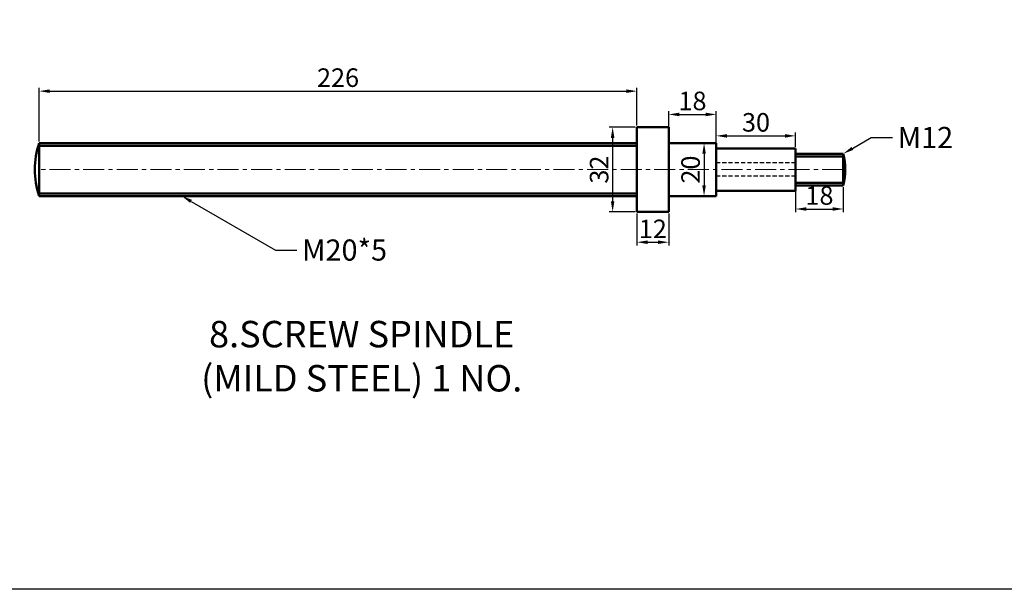
# Model space of a CAD drawing. Units: millimetres. Extents: x -66 to 1195, y -396 to 398.
# Tile 3 of 8: x 373 to 745, y -396 to -180. Entities that reach past the tile are written whole.
import ezdxf
from ezdxf import colors
from ezdxf.entities.mleader import LeaderData, LeaderLine
from ezdxf.math import Vec2, Vec3

# ---------------------------------------------------------------- set-up
doc = ezdxf.new("R2010")
doc.units = ezdxf.units.MM
doc.header["$LTSCALE"] = 0.5
doc.linetypes.add('CENTER', pattern=[50.8, 31.75, -6.35, 6.35, -6.35])
doc.linetypes.add('HIDDEN', pattern=[9.525, 6.35, -3.175])
for name, color, linetype, lineweight in [('M-CNTR', 1, 'CENTER', 18), ('M-DIMS', 2, 'Continuous', 25), ('M-HIDN', 3, 'HIDDEN', 25), ('M-OUTL', 7, 'Continuous', 50), ('M-TEXT', 7, 'Continuous', 25), ('M-TTLB', 7, 'Continuous', 25)]:
    doc.layers.add(name, color=color, linetype=linetype, lineweight=lineweight)
doc.styles.get("Standard").update_dxf_attribs({"font": 'arial.ttf'})
doc.dimstyles.new('ISO-25', dxfattribs={"dimtxt": 7, "dimasz": 4, "dimexe": 1.25, "dimexo": 0.625, "dimtad": 1, "dimtoh": 1, "dimtxsty": 'Standard', "dimcen": 2.5, "dimadec": 0, "dimazin": 0, "dimtfac": 1, "dimtmove": 0, "dimatfit": 3, "dimfxl": 1, "dimarcsym": 0})

# ---------------------------------------------------------------- blocks, each defined once
blk = doc.blocks.new('*D96')
at = {"layer": 'Defpoints', "color": 0, "ltscale": 0.5, "transparency": 16777216}
for p in [(606.02, -207.48), (606.02, -221.12), (380.02, -227.12)]:
    blk.add_point(p, dxfattribs=at)
at = {"layer": 'M-DIMS', "color": 0, "lineweight": -2, "ltscale": 0.5, "transparency": 16777216}
for p, q in [((380.02, -226.49), (380.02, -206.23)), ((384.02, -207.48), (602.02, -207.48)), ((606.02, -220.49), (606.02, -206.23))]:
    blk.add_line(p, q, dxfattribs=at)
at = {"layer": 'M-DIMS', "color": 0, "ltscale": 0.5, "transparency": 16777216}
for points in [[(384.02, -206.82), (384.02, -208.15), (380.02, -207.48)], [(602.02, -206.82), (602.02, -208.15), (606.02, -207.48)]]:
    blk.add_solid(points, dxfattribs=at)
at = {"layer": 'M-DIMS', "color": 0, "ltscale": 0.5, "transparency": 16777216, "insert": (493.02, -203.28), "char_height": 7, "attachment_point": 5}
blk.add_mtext('226', dxfattribs=at)
blk = doc.blocks.new('*D97')
at = {"layer": 'Defpoints', "color": 0, "ltscale": 0.5, "transparency": 16777216}
for p in [(606.02, -221.12), (596.83, -253.12), (606.02, -253.12)]:
    blk.add_point(p, dxfattribs=at)
at = {"layer": 'M-DIMS', "color": 0, "lineweight": -2, "ltscale": 0.5, "transparency": 16777216}
for p, q in [((605.39, -221.12), (595.58, -221.12)), ((596.83, -225.12), (596.83, -249.12)), ((605.39, -253.12), (595.58, -253.12))]:
    blk.add_line(p, q, dxfattribs=at)
at = {"layer": 'M-DIMS', "color": 0, "ltscale": 0.5, "transparency": 16777216}
for points in [[(596.17, -225.12), (597.5, -225.12), (596.83, -221.12)], [(596.17, -249.12), (597.5, -249.12), (596.83, -253.12)]]:
    blk.add_solid(points, dxfattribs=at)
at = {"layer": 'M-DIMS', "color": 0, "ltscale": 0.5, "transparency": 16777216, "insert": (592.63, -237.12), "char_height": 7, "attachment_point": 5, "rotation": 90}
blk.add_mtext('32', dxfattribs=at)
blk = doc.blocks.new('*D98')
at = {"layer": 'Defpoints', "color": 0, "ltscale": 0.5, "transparency": 16777216}
for p in [(606.02, -253.12), (618.02, -253.12), (618.02, -264.56)]:
    blk.add_point(p, dxfattribs=at)
at = {"layer": 'M-DIMS', "color": 0, "lineweight": -2, "ltscale": 0.5, "transparency": 16777216}
for p, q in [((606.02, -253.74), (606.02, -265.81)), ((618.02, -253.74), (618.02, -265.81)), ((610.02, -264.56), (614.02, -264.56))]:
    blk.add_line(p, q, dxfattribs=at)
at = {"layer": 'M-DIMS', "color": 0, "ltscale": 0.5, "transparency": 16777216}
for points in [[(610.02, -263.89), (610.02, -265.22), (606.02, -264.56)], [(614.02, -263.89), (614.02, -265.22), (618.02, -264.56)]]:
    blk.add_solid(points, dxfattribs=at)
at = {"layer": 'M-DIMS', "color": 0, "ltscale": 0.5, "transparency": 16777216, "insert": (612.02, -260.42), "char_height": 7, "attachment_point": 5}
blk.add_mtext('12', dxfattribs=at)
blk = doc.blocks.new('*D99')
at = {"layer": 'Defpoints', "color": 0, "ltscale": 0.5, "transparency": 16777216}
for p in [(627.02, -227.12), (627.02, -247.12), (631.4, -247.12)]:
    blk.add_point(p, dxfattribs=at)
at = {"layer": 'M-DIMS', "color": 0, "lineweight": -2, "ltscale": 0.5, "transparency": 16777216}
for p, q in [((627.64, -227.12), (632.65, -227.12)), ((631.4, -231.12), (631.4, -243.12)), ((627.64, -247.12), (632.65, -247.12))]:
    blk.add_line(p, q, dxfattribs=at)
at = {"layer": 'M-DIMS', "color": 0, "ltscale": 0.5, "transparency": 16777216}
for points in [[(630.73, -231.12), (632.06, -231.12), (631.4, -227.12)], [(630.73, -243.12), (632.06, -243.12), (631.4, -247.12)]]:
    blk.add_solid(points, dxfattribs=at)
at = {"layer": 'M-DIMS', "color": 0, "ltscale": 0.5, "transparency": 16777216, "insert": (627.2, -237.12), "char_height": 7, "attachment_point": 5, "rotation": 90}
blk.add_mtext('20', dxfattribs=at)
blk = doc.blocks.new('*D100')
at = {"layer": 'Defpoints', "color": 0, "ltscale": 0.5, "transparency": 16777216}
for p in [(636.02, -216.28), (618.02, -227.12), (636.02, -227.12)]:
    blk.add_point(p, dxfattribs=at)
at = {"layer": 'M-DIMS', "color": 0, "lineweight": -2, "ltscale": 0.5, "transparency": 16777216}
for p, q in [((618.02, -226.49), (618.02, -215.03)), ((636.02, -226.49), (636.02, -215.03)), ((622.02, -216.28), (632.02, -216.28))]:
    blk.add_line(p, q, dxfattribs=at)
at = {"layer": 'M-DIMS', "color": 0, "ltscale": 0.5, "transparency": 16777216}
for points in [[(622.02, -215.61), (622.02, -216.94), (618.02, -216.28)], [(632.02, -215.61), (632.02, -216.94), (636.02, -216.28)]]:
    blk.add_solid(points, dxfattribs=at)
at = {"layer": 'M-DIMS', "color": 0, "ltscale": 0.5, "transparency": 16777216, "insert": (627.02, -212.08), "char_height": 7, "attachment_point": 5}
blk.add_mtext('18', dxfattribs=at)
blk = doc.blocks.new('*D101')
at = {"layer": 'Defpoints', "color": 0, "ltscale": 0.5, "transparency": 16777216}
for p in [(666.02, -224.37), (636.02, -229.12), (666.02, -229.12)]:
    blk.add_point(p, dxfattribs=at)
at = {"layer": 'M-DIMS', "color": 0, "lineweight": -2, "ltscale": 0.5, "transparency": 16777216}
for p, q in [((636.02, -228.49), (636.02, -223.12)), ((666.02, -228.49), (666.02, -223.12)), ((640.02, -224.37), (662.02, -224.37))]:
    blk.add_line(p, q, dxfattribs=at)
at = {"layer": 'M-DIMS', "color": 0, "ltscale": 0.5, "transparency": 16777216}
for points in [[(640.02, -223.71), (640.02, -225.04), (636.02, -224.37)], [(662.02, -223.71), (662.02, -225.04), (666.02, -224.37)]]:
    blk.add_solid(points, dxfattribs=at)
at = {"layer": 'M-DIMS', "color": 0, "ltscale": 0.5, "transparency": 16777216, "insert": (651.02, -220.17), "char_height": 7, "attachment_point": 5}
blk.add_mtext('30', dxfattribs=at)
blk = doc.blocks.new('*D102')
at = {"layer": 'Defpoints', "color": 0, "ltscale": 0.5, "transparency": 16777216}
for p in [(666.02, -243.12), (684.02, -243.12), (684.02, -252.01)]:
    blk.add_point(p, dxfattribs=at)
at = {"layer": 'M-DIMS', "color": 0, "lineweight": -2, "ltscale": 0.5, "transparency": 16777216}
for p, q in [((666.02, -243.74), (666.02, -253.26)), ((684.02, -243.74), (684.02, -253.26)), ((670.02, -252.01), (680.02, -252.01))]:
    blk.add_line(p, q, dxfattribs=at)
at = {"layer": 'M-DIMS', "color": 0, "ltscale": 0.5, "transparency": 16777216}
for points in [[(670.02, -251.34), (670.02, -252.68), (666.02, -252.01)], [(680.02, -251.34), (680.02, -252.68), (684.02, -252.01)]]:
    blk.add_solid(points, dxfattribs=at)
at = {"layer": 'M-DIMS', "color": 0, "ltscale": 0.5, "transparency": 16777216, "insert": (675.02, -247.81), "char_height": 7, "attachment_point": 5}
blk.add_mtext('18', dxfattribs=at)

msp = doc.modelspace()

# ---------------------------------------------------------------- linework, layer by layer
at = {"layer": 'M-CNTR', "ltscale": 0.5}
msp.add_line((684.016, -237.1162), (380.016, -237.1162), dxfattribs=at)
at = {"layer": 'M-HIDN', "ltscale": 0.5}
for p, q in [((666.016, -234.6162), (636.016, -234.6162)), ((666.016, -239.6162), (636.016, -239.6162))]:
    msp.add_line(p, q, dxfattribs=at)
at = {"layer": 'M-OUTL', "ltscale": 0.5}
for p, q in [((606.016, -221.1162), (606.016, -253.1162)), ((618.016, -221.1162), (606.016, -221.1162)), ((618.016, -253.1162), (618.016, -221.1162)), ((380.016, -227.1162), (606.016, -227.1162)), ((380.016, -247.1162), (380.016, -227.1162)), ((380.016, -228.1162), (606.016, -228.1162)), ((606.016, -227.1162), (606.016, -247.1162)), ((618.016, -227.1162), (636.016, -227.1162)), ((618.016, -247.1162), (618.016, -227.1162)), ((636.016, -227.1162), (636.016, -247.1162)), ((636.016, -229.1162), (666.016, -229.1162)), ((636.016, -245.1162), (636.016, -229.1162)), ((666.016, -229.1162), (666.016, -245.1162)), ((666.016, -231.1162), (684.016, -231.1162)), ((666.016, -243.1162), (666.016, -231.1162)), ((666.016, -232.1162), (684.016, -232.1162)), ((684.016, -231.1162), (684.016, -243.1162)), ((666.016, -245.1162), (636.016, -245.1162)), ((684.016, -242.1162), (666.016, -242.1162)), ((684.016, -243.1162), (666.016, -243.1162)), ((606.016, -246.1162), (380.016, -246.1162)), ((606.016, -247.1162), (380.016, -247.1162)), ((636.016, -247.1162), (618.016, -247.1162)), ((606.016, -253.1162), (618.016, -253.1162))]:
    msp.add_line(p, q, dxfattribs=at)
for centre, radius, start, end in [((410.0673, -237.1162), 31.6715, 161.59443, 198.40557), ((660.1049, -237.1162), 24.6523, 345.913611, 14.086389)]:
    msp.add_arc(centre, radius, start, end, dxfattribs=at)
at = {"layer": 'M-TTLB', "ltscale": 0.5}
msp.add_lwpolyline([(-66.4176, 397.641), (1195.0519, 397.641), (1195.0519, -395.6964), (-66.4176, -395.6964)], close=True, dxfattribs=at)

# ---------------------------------------------------------------- texts
at = {"layer": 'M-TEXT', "ltscale": 0.5, "insert": (399.9608, -294.2857), "char_height": 10, "attachment_point": 1}
msp.add_mtext_dynamic_manual_height_columns('\\pxqc;8.SCREW SPINDLE \\P(MILD STEEL) 1 NO.', width=203.992441, gutter_width=12.5, heights=[0], dxfattribs=at)

# ---------------------------------------------------------------- dimensions: what is measured, and where the dimension line sits
at = {"layer": 'M-DIMS', "ltscale": 0.5}
for base, p1, p2, picture, middle in [((606.016, -207.4818), (380.016, -227.1162), (606.016, -221.1162), '*D96', (493.016, -203.2828)), ((636.016, -216.2767), (618.016, -227.1162), (636.016, -227.1162), '*D100', (627.016, -212.0777)), ((666.016, -224.3743), (636.016, -229.1162), (666.016, -229.1162), '*D101', (651.016, -220.1729)), ((684.016, -252.0088), (666.016, -243.1162), (684.016, -243.1162), '*D102', (675.016, -247.8097)), ((618.016, -264.5562), (606.016, -253.1162), (618.016, -253.1162), '*D98', (612.016, -260.4169))]:
    dim = msp.add_linear_dim(base=base, p1=p1, p2=p2, dimstyle='ISO-25', override={"dimclrd": 0, "dimclre": 0, "dimclrt": 0}, dxfattribs=at)
    dim.commit()
    dim.dimension.update_dxf_attribs({"geometry": picture, "text_midpoint": middle})
for base, p1, p2, picture, middle in [((596.8332, -253.1162), (606.016, -221.1162), (606.016, -253.1162), '*D97', (592.6318, -237.1162)), ((631.3954, -247.1162), (627.016, -227.1162), (627.016, -247.1162), '*D99', (627.1964, -237.1162))]:
    dim = msp.add_linear_dim(base=base, p1=p1, p2=p2, angle=90, dimstyle='ISO-25', override={"dimclrd": 0, "dimclre": 0, "dimclrt": 0}, dxfattribs=at)
    dim.commit()
    dim.dimension.update_dxf_attribs({"geometry": picture, "text_midpoint": middle})

# ---------------------------------------------------------------- leaders
at = {"layer": 'M-TEXT', "ltscale": 0.5}
ml = msp.add_multileader_mtext('Standard', dxfattribs=at)
ml.set_content('M12', color=256)
ml.set_leader_properties()
ml.build(insert=Vec2(0, 0))
ctx = ml.context
ctx.base_point, ctx.char_height, ctx.plane_origin = Vec3(702.598, -225.0067), 8, Vec3(684.016, -231.1162)
notes = []
notes.append((ctx, [(0, (1, 1, 0), (694.598, -225.0067), (1, 0), 8, [(0, [(684.016, -231.1162)], 0, [])])]))
ctx.mtext.insert, ctx.mtext.flow_direction = Vec3(704.598, -221.0067), 5
ml = msp.add_multileader_mtext('Standard', dxfattribs=at)
ml.set_content('M20*5', color=256)
ml.set_leader_properties()
ml.build(insert=Vec2(0, 0))
ctx = ml.context
ctx.base_point, ctx.char_height, ctx.plane_origin = Vec3(477.422, -267.5842), 8, Vec3(433.9703, -247.1162)
notes.append((ctx, [(0, (1, 1, 0), (469.422, -267.5842), (1, 0), 8, [(0, [(433.9703, -247.1162)], 0, [])])]))
ctx.mtext.insert, ctx.mtext.flow_direction = Vec3(479.422, -263.516), 5
for ctx, leaders in notes:
    for number, flags, end, landing, length, lines in leaders:
        leader = LeaderData()
        leader.index, (leader.has_last_leader_line, leader.has_dogleg_vector, leader.attachment_direction) = number, flags
        leader.last_leader_point, leader.dogleg_vector, leader.dogleg_length = Vec3(end), Vec3(landing), length
        for number, points, colour, breaks in lines:
            line = LeaderLine()
            line.index, line.vertices, line.color, line.breaks = number, Vec3.list(points), colors.encode_raw_color(colour), breaks
            leader.lines.append(line)
        ctx.leaders.append(leader)

doc.saveas('drawing.dxf')
